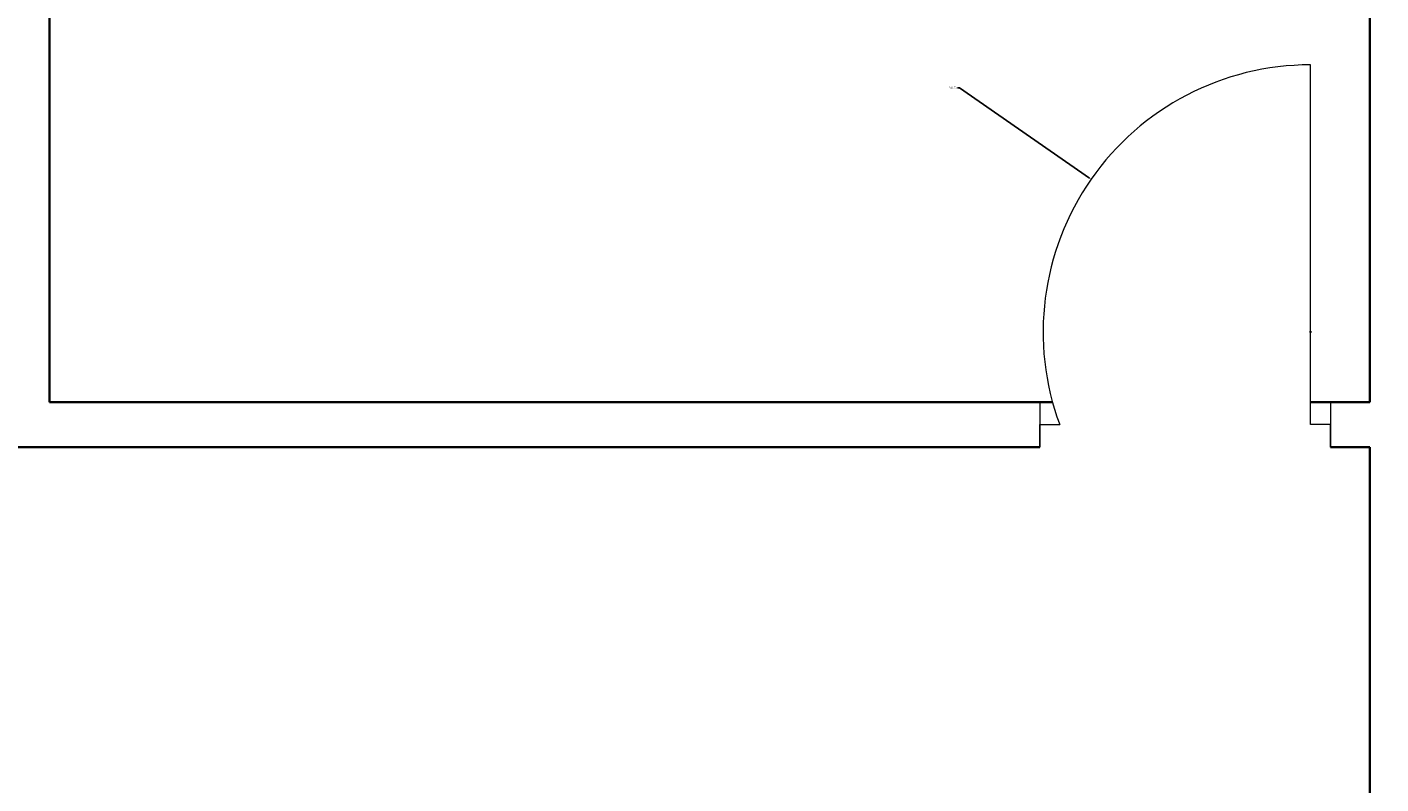
# Model space of a CAD drawing. Units: inches. Extents: x 2163 to 2982, y 1024 to 2288.
# Tile 17 of 22: x 2448 to 2583, y 1978 to 2054. Entities that reach past the tile are written whole.
import ezdxf

# ---------------------------------------------------------------- set-up
doc = ezdxf.new("R2010")
doc.units = ezdxf.units.IN
for name, color, linetype, lineweight in [('A-ANNO-DIMS', 2, 'Continuous', 18), ('A-DOOR', 11, 'Continuous', 18), ('A-WALL', 7, 'Continuous', 35)]:
    doc.layers.add(name, color=color, linetype=linetype, lineweight=lineweight)
doc.styles.get("Standard").update_dxf_attribs({"font": 'arial.ttf'})
doc.dimstyles.get("Standard").update_dxf_attribs({"dimtxt": 0.18, "dimasz": 0.18, "dimexe": 0.18, "dimexo": 0.0625, "dimgap": 0.09, "dimtad": 0, "dimtih": 1, "dimtoh": 1, "dimdec": 4, "dimzin": 0, "dimdsep": 46, "dimtxsty": 'Standard', "dimcen": 0.09, "dimadec": 0, "dimazin": 0, "dimtfac": 1, "dimtdec": 4, "dimtofl": 0, "dimtmove": 0, "dimatfit": 3, "dimfxl": 1, "dimtolj": 1, "dimtzin": 0, "dimarcsym": 0})

# ---------------------------------------------------------------- blocks, each defined once
blk = doc.blocks.new('*D29')
at = {"layer": 'A-ANNO-DIMS', "color": 0, "lineweight": -2, "transparency": 16777216}
for p, q in [((2285.34, 1738.83), (2285.34, 2288.1)), ((2285.52, 2287.92), (2576.05, 2287.92)), ((2867.16, 2287.92), (2576.63, 2287.92)), ((2867.34, 2229.33), (2867.34, 2288.1))]:
    blk.add_line(p, q, dxfattribs=at)
at = {"layer": 'A-ANNO-DIMS', "color": 0, "transparency": 16777216}
for points in [[(2285.52, 2287.95), (2285.52, 2287.89), (2285.34, 2287.92)], [(2867.16, 2287.95), (2867.16, 2287.89), (2867.34, 2287.92)]]:
    blk.add_solid(points, dxfattribs=at)
at = {"layer": 'Defpoints', "color": 0, "transparency": 16777216}
for p in [(2867.34, 2287.92), (2867.34, 2229.27), (2285.34, 1738.77)]:
    blk.add_point(p, dxfattribs=at)
at = {"layer": 'A-ANNO-DIMS', "color": 0, "transparency": 16777216, "insert": (2576.34, 2287.92), "char_height": 0.18, "attachment_point": 5}
blk.add_mtext('\\A1;582', dxfattribs=at)
blk = doc.blocks.new('*D49')
at = {"layer": 'A-ANNO-DIMS', "color": 0, "lineweight": -2, "transparency": 16777216}
for p, q in [((2541.14, 2047.73), (2541.32, 2047.73)), ((2541.32, 2047.73), (2554.33, 2038.67)), ((2576.33, 2023.29), (2576.51, 2023.29)), ((2576.42, 2023.2), (2576.42, 2023.38))]:
    blk.add_line(p, q, dxfattribs=at)
at = {"layer": 'A-ANNO-DIMS', "color": 0, "transparency": 16777216}
blk.add_solid([(2554.35, 2038.69), (2554.32, 2038.64), (2554.48, 2038.57)], dxfattribs=at)
at = {"layer": 'Defpoints', "color": 0, "transparency": 16777216}
for p in [(2554.48, 2038.57), (2576.42, 2023.29)]:
    blk.add_point(p, dxfattribs=at)
at = {"layer": 'A-ANNO-DIMS', "color": 0, "transparency": 16777216, "insert": (2540.66, 2047.73), "char_height": 0.18, "attachment_point": 5}
blk.add_mtext('\\A1;R26.73', dxfattribs=at)

msp = doc.modelspace()

# ---------------------------------------------------------------- linework, layer by layer
at = {"layer": 'A-DOOR'}
for p, q in [((2576.4158, 2014.0188), (2576.4158, 2050.0188)), ((2549.3415, 2016.2688), (2549.3415, 2011.7688)), ((2578.4158, 2016.2688), (2578.4158, 2011.7688)), ((2549.3415, 2011.7688), (2549.3415, 2014.0188)), ((2549.3415, 2014.0188), (2551.3415, 2014.0188)), ((2578.4158, 2014.0188), (2576.4158, 2014.0188)), ((2578.4158, 2011.7688), (2578.4158, 2014.0188))]:
    msp.add_line(p, q, dxfattribs=at)
msp.add_arc((2576.4158, 2023.2866), 26.7322, 90, 200.284923, dxfattribs=at)
at = {"layer": 'A-WALL'}
for p, q in [((2450.3389, 2172.2688), (2450.3389, 2016.2688)), ((2582.3389, 2172.2688), (2582.3389, 2016.2688)), ((2450.3389, 2016.2688), (2550.6212, 2016.2688)), ((2576.4158, 2016.2688), (2582.3389, 2016.2688)), ((2444.5397, 2011.7688), (2450.3389, 2011.7688)), ((2450.3389, 2011.7688), (2549.3415, 2011.7688)), ((2578.4158, 2011.7688), (2582.3389, 2011.7688)), ((2582.3389, 2011.7688), (2582.3389, 1738.7688))]:
    msp.add_line(p, q, dxfattribs=at)

# ---------------------------------------------------------------- dimensions: what is measured, and where the dimension line sits
at = {"layer": 'A-ANNO-DIMS'}
dim = msp.add_linear_dim(base=(2867.3389, 2287.9188), p1=(2285.3389, 1738.7688), p2=(2867.3389, 2229.2688), dimstyle='Standard', override={"dimdec": 0, "dimlfac": 1, "dimrnd": 0, "dimzin": 0, "dimdsep": 46, "dimlunit": 2}, dxfattribs=at)
dim.commit()
dim.dimension.update_dxf_attribs({"geometry": '*D29', "text_midpoint": (2576.3389, 2287.9188)})
dim = msp.add_radius_dim(center=(2576.4158, 2023.2866), mpoint=(2554.48, 2038.565), dimstyle='Standard', override={"dimdec": 2, "dimlfac": 1, "dimrnd": 0, "dimzin": 0, "dimdsep": 46, "dimlunit": 2}, dxfattribs=at)
dim.commit()
dim.dimension.update_dxf_attribs({"geometry": '*D49', "text_midpoint": (2540.6586, 2047.7321), "dimtype": 164})

doc.saveas('drawing.dxf')
